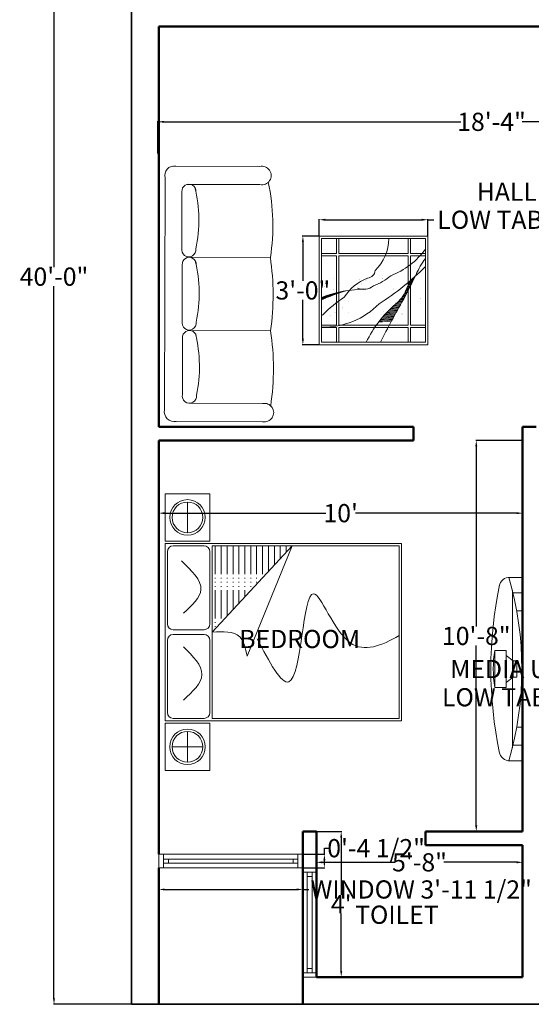
# Model space of a CAD drawing. Units: inches. Extents: x 134 to 568, y 15 to 554.
# Tile 1 of 7: x 134 to 303, y 45 to 369. Entities that reach past the tile are written whole.
import ezdxf

# ---------------------------------------------------------------- set-up
doc = ezdxf.new("R2010")
doc.units = ezdxf.units.IN
doc.header["$MEASUREMENT"] = 0
for name, color, linetype, lineweight in [('A-ANNO-DIMS', 2, 'Continuous', 18), ('A-AREA-IDEN', 7, 'Continuous', 25), ('A-EQPM', 8, 'Continuous', 18), ('A-FURN', 9, 'Continuous', 18), ('A-GLAZ', 4, 'Continuous', 18), ('A-WALL', 7, 'Continuous', 50), ('C-PROP', 7, 'Continuous', 35)]:
    doc.layers.add(name, color=color, linetype=linetype, lineweight=lineweight)
doc.styles.get("Standard").update_dxf_attribs({"font": 'arial.ttf'})
doc.dimstyles.get("Standard").update_dxf_attribs({"dimtxt": 6, "dimasz": 2, "dimexe": 0.18, "dimexo": 0.0625, "dimgap": 0.09, "dimtad": 0, "dimtih": 1, "dimtoh": 1, "dimdec": 0, "dimzin": 0, "dimdsep": 46, "dimlunit": 4, "dimtxsty": 'Standard', "dimcen": 0.09, "dimadec": 0, "dimazin": 0, "dimtfac": 1, "dimtdec": 0, "dimtofl": 0, "dimtmove": 0, "dimatfit": 3, "dimfxl": 1, "dimtolj": 1, "dimtzin": 0, "dimarcsym": 0})

# ---------------------------------------------------------------- blocks, each defined once
blk = doc.blocks.new('fdgchj')
for p, q in [((180.0833573093669, -8.682097346214732), (180.0833573093669, -13.18209734621473)), ((180.0833573093669, -8.682097346214732), (227.5833573093669, -8.682097346214716)), ((181.6833573093668, -8.682097346214732), (181.6833573093668, -13.18209734621473)), ((225.9833573093669, -8.682097346214716), (225.9833573093669, -13.18209734621463)), ((227.5833573093669, -8.682097346214716), (227.5833573093669, -13.18209734621463)), ((181.6833573093668, -10.28209734621472), (225.9833573093669, -10.28209734621471)), ((181.6833573093668, -11.58209734621473), (225.9833573093669, -11.58209734621464)), ((183.2833573093669, -10.28209734621472), (183.2833573093669, -11.58209734621473)), ((224.3833573093669, -10.28209734621471), (224.3833573093669, -11.58209734621464)), ((180.0833573093669, -13.18209734621473), (227.5833573093669, -13.18209734621463))]:
    blk.add_line(p, q)
blk = doc.blocks.new('*D9')
at = {"layer": 'A-ANNO-DIMS', "color": 0, "lineweight": -2, "transparency": 16777216}
for p, q in [((232.145857309367, 101.5821619144604), (240.4398249294156, 101.5821619144604)), ((240.2598249294155, 99.58216191446044), (240.2598249294155, 80.67216191446046)), ((240.2598249294156, 55.58216191446049), (240.2598249294155, 74.49216191446045)), ((232.1458573093669, 53.58216191446047), (240.4398249294156, 53.58216191446048))]:
    blk.add_line(p, q, dxfattribs=at)
at = {"layer": 'A-ANNO-DIMS', "color": 0, "transparency": 16777216}
for points in [[(239.9264915960822, 99.58216191446044), (240.5931582627489, 99.58216191446044), (240.2598249294155, 101.5821619144604)], [(239.9264915960822, 55.58216191446048), (240.5931582627489, 55.58216191446049), (240.2598249294156, 53.58216191446048)]]:
    blk.add_solid(points, dxfattribs=at)
at = {"layer": 'Defpoints', "color": 0, "transparency": 16777216}
for p in [(232.083357309367, 101.5821619144604), (232.0833573093669, 53.58216191446047), (240.2598249294156, 53.58216191446048)]:
    blk.add_point(p, dxfattribs=at)
at = {"layer": 'A-ANNO-DIMS', "color": 0, "transparency": 16777216, "insert": (240.2598249294155, 77.58216191446037), "char_height": 6, "attachment_point": 5}
blk.add_mtext("\\A1;4'", dxfattribs=at)
blk = doc.blocks.new('*D14')
at = {"layer": 'A-ANNO-DIMS', "color": 0, "lineweight": -2, "transparency": 16777216}
for p, q in [((300.0208573093672, 230.5821619144605), (284.6214758231763, 230.5821619144605)), ((284.8014758231764, 228.5821619144605), (284.8014758231764, 169.2355998407906)), ((284.8014758231764, 103.5821619144604), (284.8014758231764, 162.9287239881303)), ((300.020857309367, 101.5821619144604), (284.6214758231764, 101.5821619144604))]:
    blk.add_line(p, q, dxfattribs=at)
at = {"layer": 'A-ANNO-DIMS', "color": 0, "transparency": 16777216}
for points in [[(284.4681424898431, 228.5821619144605), (285.1348091565096, 228.5821619144605), (284.8014758231764, 230.5821619144605)], [(284.4681424898431, 103.5821619144604), (285.1348091565098, 103.5821619144604), (284.8014758231764, 101.5821619144604)]]:
    blk.add_solid(points, dxfattribs=at)
at = {"layer": 'Defpoints', "color": 0, "transparency": 16777216}
for p in [(300.0833573093672, 230.5821619144605), (284.8014758231764, 101.5821619144604), (300.083357309367, 101.5821619144604)]:
    blk.add_point(p, dxfattribs=at)
at = {"layer": 'A-ANNO-DIMS', "color": 0, "transparency": 16777216, "insert": (284.8014758231764, 166.0821619144603), "char_height": 6, "attachment_point": 5}
blk.add_mtext('\\A1;10\'-8"', dxfattribs=at)
blk = doc.blocks.new('*D15')
at = {"layer": 'A-ANNO-DIMS', "color": 0, "lineweight": -2, "transparency": 16777216}
for p, q in [((180.0833573093669, 230.5196619144604), (180.0833573093669, 206.3961685645716)), ((300.0833573093669, 230.5196619144604), (300.0833573093669, 206.3961685645716)), ((182.0833573093669, 206.5761685645716), (235.1843532165974, 206.5761685645716)), ((298.0833573093669, 206.5761685645716), (244.9823614021363, 206.5761685645716))]:
    blk.add_line(p, q, dxfattribs=at)
at = {"layer": 'A-ANNO-DIMS', "color": 0, "transparency": 16777216}
for points in [[(182.0833573093669, 206.909501897905), (182.0833573093669, 206.2428352312383), (180.0833573093669, 206.5761685645716)], [(298.0833573093669, 206.909501897905), (298.0833573093669, 206.2428352312383), (300.0833573093669, 206.5761685645716)]]:
    blk.add_solid(points, dxfattribs=at)
at = {"layer": 'Defpoints', "color": 0, "transparency": 16777216}
for p in [(180.0833573093669, 230.5821619144603), (300.0833573093669, 230.5821619144603), (300.0833573093669, 206.5761685645716)]:
    blk.add_point(p, dxfattribs=at)
at = {"layer": 'A-ANNO-DIMS', "color": 0, "transparency": 16777216, "insert": (240.0833573093669, 206.5761685645716), "char_height": 6, "attachment_point": 5}
blk.add_mtext("\\A1;10'", dxfattribs=at)
blk = doc.blocks.new('*D22')
at = {"layer": 'A-ANNO-DIMS', "color": 0, "lineweight": -2, "transparency": 16777216}
for p, q in [((179.8333573093669, 325.1446619144604), (179.8333573093669, 335.8252549678748)), ((181.8333573093669, 335.6452549678747), (279.7201649492031, 335.6452549678747)), ((397.8333573093669, 335.6452549678747), (299.9465496695306, 335.6452549678747)), ((399.8333573093669, 325.1446619144604), (399.8333573093669, 335.8252549678748))]:
    blk.add_line(p, q, dxfattribs=at)
at = {"layer": 'A-ANNO-DIMS', "color": 0, "transparency": 16777216}
for points in [[(181.8333573093669, 335.978588301208), (181.8333573093669, 335.3119216345414), (179.8333573093669, 335.6452549678747)], [(397.8333573093669, 335.978588301208), (397.8333573093669, 335.3119216345414), (399.8333573093669, 335.6452549678747)]]:
    blk.add_solid(points, dxfattribs=at)
at = {"layer": 'Defpoints', "color": 0, "transparency": 16777216}
for p in [(179.8333573093669, 335.6452549678747), (179.8333573093669, 325.0821619144604), (399.8333573093669, 325.0821619144604)]:
    blk.add_point(p, dxfattribs=at)
at = {"layer": 'A-ANNO-DIMS', "color": 0, "transparency": 16777216, "insert": (289.8333573093669, 335.6452549678747), "char_height": 6, "attachment_point": 5}
blk.add_mtext('\\A1;18\'-4"', dxfattribs=at)
blk = doc.blocks.new('dfghj')
h = blk.add_hatch()
h.set_pattern_fill('ACAD_ISO06W100', color=256, scale=0.5400000000000001, style=0)
h.set_pattern_definition([(0, (-45.65929459918516, 81.2680393364767), (0, 2.7), [12.96, -1.62, 0.27, -1.62, 0.27, -3.51]), (0, (-45.65929459918516, 81.2680393364767), (0, 2.7), [-18.36, 0.27, -1.62])])
h.paths.add_polyline_path([(495.420705400802, 683.3680393364771), (534.8407054008148, 646.8981935885663), (534.8407054008148, 683.3680393364771)])
for p, q in [((432.2407054008163, 704.9680393364765), (453.8407054008148, 704.9680393364765)), ((432.2407054008163, 704.9680393364765), (432.2407054008163, 684.4480393364788)), ((443.0407054008119, 701.7280393364721), (443.0407054008119, 687.6880393364768)), ((453.8407054008148, 704.9680393364765), (453.8407054008148, 684.4480393364788)), ((454.920705400802, 704.9680393364765), (454.920705400802, 596.9680393364765)), ((454.920705400802, 704.9680393364765), (535.920705400802, 704.9680393364765)), ((458.7007054008154, 703.8880393364766), (491.6407054008105, 703.8880393364766)), ((499.2007054008154, 703.8880393364766), (532.1407054008104, 703.8880393364766)), ((535.920705400802, 704.9680393364765), (535.920705400802, 596.9680393364765)), ((537.0007054008183, 704.9680393364765), (558.6007054008168, 704.9680393364765)), ((537.0007054008183, 704.9680393364765), (537.0007054008183, 684.4480393364788)), ((558.6007054008168, 704.9680393364765), (558.6007054008168, 684.4480393364788)), ((456.0007054008183, 701.1880393364767), (456.0007054008183, 687.1480393364795)), ((494.3407054008148, 701.1880393364767), (494.3407054008148, 687.1480393364795)), ((496.5007054008183, 701.1880393364767), (496.5007054008183, 687.1480393364795)), ((534.8407054008148, 701.1880393364767), (534.8407054008148, 687.1480393364795)), ((436.0207054008006, 694.7080393364744), (450.060705400816, 694.7080393364744)), ((540.7807054008099, 694.7080393364744), (554.8207054008035, 694.7080393364744)), ((432.2407054008163, 684.4480393364788), (453.8407054008148, 684.4480393364788)), ((458.7007054008154, 684.4480393364788), (491.6407054008105, 684.4480393364788)), ((499.2007054008154, 684.4480393364788), (532.1407054008104, 684.4480393364788)), ((537.0007054008183, 684.4480393364788), (558.6007054008168, 684.4480393364788)), ((456.0007054008183, 683.3680393364771), (456.0007054008183, 598.0480393364792)), ((456.0007054008183, 683.3680393364771), (534.8407054008148, 683.3680393364771)), ((495.420705400802, 683.3680393364771), (534.8407054008148, 646.8981935885663)), ((534.8407054008148, 683.3680393364771), (534.8407054008148, 598.0480393364792)), ((484.408206427508, 667.4334197787679), (534.8407054008148, 646.8981935885663)), ((456.0007054008183, 598.0480393364792), (534.8407054008148, 598.0480393364792)), ((454.920705400802, 596.9680393364765), (535.920705400802, 596.9680393364765))]:
    blk.add_line(p, q)
for centre, radius in [((443.0407054008119, 694.7080393364744), 8.1), ((443.0407054008119, 694.7080393364744), 7.020000000000001), ((547.800705400814, 694.7080393364744), 8.1), ((547.800705400814, 694.7080393364744), 7.020000000000001)]:
    blk.add_circle(centre, radius)
for centre, start, end in [((458.7007054008154, 701.1880393364767), 90, 180), ((491.6407054008105, 701.1880393364767), 0, 90), ((499.2007054008154, 701.1880393364767), 90, 180), ((532.1407054008104, 701.1880393364767), 0, 90), ((458.7007054008154, 687.1480393364795), 180, 270), ((491.6407054008105, 687.1480393364795), 270, 0), ((499.2007054008154, 687.1480393364795), 180, 270), ((532.1407054008104, 687.1480393364795), 270, 0)]:
    blk.add_arc(centre, 2.7, start, end)
for points, knots in [([(504.0873642108144, 696.4980886587387), (507.6478568661273, 692.6728528270118), (515.4209753861596, 684.3217580865917), (523.5337025619604, 692.8242520545471), (527.9303786509863, 697.4321614684745)], [0, 0, 0, 0, 13.36633595571319, 29.18082513308789, 29.18082513308789, 29.18082513308789, 29.18082513308789]), ([(464.3490068105038, 696.4980886587387), (468.2209746909002, 692.3657909551906), (476.1716983091387, 683.8805044125166), (484.4253643000896, 692.2199280984504), (488.6595307904953, 696.4980886587387)], [0, 0, 0, 0, 14.39706672085805, 29.56302891623292, 29.56302891623292, 29.56302891623292, 29.56302891623292]), ([(484.408206427508, 667.4334197787679), (487.9117447952648, 668.1466020798161), (496.0584065288031, 669.8049412646973), (495.6522124186928, 678.4441772793408), (495.420705400802, 683.3680393364771)], [0, 0, 0, 0, 9.565159985887036, 22.24154972850861, 22.24154972850861, 22.24154972850861, 22.24154972850861]), ([(492.399610210059, 662.8714304071177), (481.8503788042744, 657.380170521003), (453.252508497726, 642.4939354956872), (538.2357400049532, 642.1800857884786), (482.0018716074937, 623.4329456516238), (489.252723434607, 606.1225063401602), (493.8220791548028, 598.0480393364792)], [0, 0, 0, 0, 451.7784176077852, 1224.72435166985, 1743.990776893513, 2173.853229184429, 2173.853229184429, 2173.853229184429, 2173.853229184429])]:
    blk.add_open_spline(points, degree=3, knots=knots)
blk = doc.blocks.new('A$C78AE5658')
for p, q in [((1514.710072450669, 306.1060037219359), (1514.710072450669, 524.1059474034627)), ((1514.710072450669, 524.1059474034627), (2235.5102586675, 524.1059474034627)), ((2235.5102586675, 306.1060037219359), (2235.5102586675, 524.1059474034627)), ((98.35715676363363, 250.0000009555879), (98.35715676363363, 251.6199660723724)), ((98.35715676367727, 250.0000009555733), (98.35715676361907, 9.555878933e-07)), ((1514.710072450669, 306.1060037219359), (2235.5102586675, 306.1060037219359)), ((1613.280102290542, 306.1060037219359), (1715.729798347087, 167.9763742110153)), ((2136.940228827627, 306.1060037219359), (2034.490532771082, 167.9763742110153)), ((3648.35715676359, 250.0000009555733), (3648.35715676359, 251.6199660720231)), ((3648.35715676359, 9.555733413e-07), (3648.35715676359, 250.0000009555733)), ((3648.357156763605, 9.555733413e-07), (98.35715676363363, 9.555878933e-07)), ((348.3571567636482, 183.569161564541), (3398.357156763547, 183.5691615645264)), ((398.3571567636482, 9.555733413e-07), (398.3571567636482, 171.5666306721468)), ((748.357156763648, 9.555733413e-07), (748.357156763648, 99.2393274621354)), ((2034.490532771082, 167.9763742110153), (1715.729425914915, 167.9763742110153)), ((1715.729425914915, 167.9763742110153), (1715.729425914915, 97.54311758768019)), ((2034.490532771082, 97.54311758768019), (1715.729425914915, 97.54311758768019)), ((2034.490532771082, 167.9763742110153), (2034.490532771082, 97.54311758768019)), ((2998.35715676359, 9.555733413e-07), (2998.35715676359, 99.2393274621354)), ((3348.35715676359, 9.555733413e-07), (3348.35715676359, 171.5666306721468))]:
    blk.add_line(p, q)
blk.add_lwpolyline([(246.4015375078543, 431.9827464358895, -0.103184122095167), (3500.312775983877, 431.9827464432965, -0.103184122095167)], format="xyb")
for centre, radius, start, end in [((297.9418522906435, 238.7378345952966), 200, 98.46874505780073, 183.6930153877844), ((1875.110165559085, -1674.917347937364), 2228.360760865037, 80.69248372113285, 99.30751627886714), ((3448.772461236565, 238.7378345952966), 200, 356.3069846122155, 81.53125494219925), ((1873.357156763633, 6426.250000955618), 6426.25000000003, 253.9658138527447, 286.0341861472553)]:
    blk.add_arc(centre, radius, start, end)
blk = doc.blocks.new('A$C25EC1EFB')
h = blk.add_hatch()
h.set_pattern_fill('ANSI31', color=256, scale=2.508, angle=580, style=0)
h.set_pattern_definition([(94.99999999999984, (2801.512250582819, 4289.79602251789), (7.93259876143476, 0.6940124639253284), [])])
edge = h.paths.add_edge_path()
edge.add_ellipse((4084.490467177063, -2815.580363917667), major_axis=(-3872.16408689083, 3872.16408689083), ratio=0.9999999999995552, start_angle=340.89961915580596, end_angle=343.15488567038426, ccw=False)
edge.add_ellipse((1486.624568246823, 2293.159848771007), major_axis=(-194.6618757392838, 194.6618757392838), ratio=0.9999999999999246, start_angle=154.9056197196584, end_angle=183.4247301497222, ccw=False)
edge.add_ellipse((1687.117678346121, 1762.501521206774), major_axis=(-206.4950185728816, 206.4950185728816), ratio=0.999999999999898, start_angle=-23.5559095241906, end_angle=5.886608761987814)
edge.add_ellipse((823.8605303866296, 2467.162105106873), major_axis=(-581.4647167234576, 581.4647167234575), ratio=0.9999999999998493, start_angle=171.3363574034995, end_angle=185.7365630084011, ccw=False)
edge.add_line((1311.102457978037, 1804.744006331188), (1311.102457978037, 1908.515397835807))
edge.add_ellipse((-1407.416444189095, 7084.924681207201), major_axis=(4134.341428234145, 4134.341428234145), ratio=0.9999999999998351, start_angle=252.7073165240117, end_angle=254.8255249662156)
for p, q in [((1118.231915589249, 2219.932055225661), (1118.231915589242, 1300.332055225655)), ((2037.831915589246, 2219.932055225647), (1118.231915589249, 2219.932055225661)), ((2016.931915589244, 2199.032055225638), (1139.131915589243, 2199.032055225638)), ((1139.131915589243, 2199.032055225638), (1139.131915589243, 1321.232055225664)), ((1264.531915589245, 2199.032055225638), (1264.531915589245, 2073.63205522563)), ((1285.431915589246, 2199.032055225638), (1285.431915589246, 2073.63205522563)), ((1870.631915589243, 2199.032055225638), (1870.631915589243, 2073.632055225644)), ((1891.531915589245, 2199.032055225638), (1891.531915589245, 2073.632055225644)), ((2016.931915589244, 2199.032055225638), (2016.931915589244, 1321.23205522565)), ((2037.831915589246, 2219.932055225647), (2037.831915589246, 1300.332055225655)), ((1264.531915589245, 2073.63205522563), (1139.131915589243, 2073.632055225644)), ((1264.531915589245, 2052.732055225635), (1139.131915589243, 2052.732055225664)), ((1264.531915589245, 2052.732055225635), (1264.531915589245, 1467.532055225652)), ((1870.631915589243, 2073.632055225644), (1285.431915589246, 2073.63205522563)), ((1870.631915589243, 2052.73205522565), (1285.431915589246, 2052.732055225635)), ((1285.431915589246, 2052.732055225635), (1285.431915589246, 1467.532055225652)), ((1870.631915589243, 2052.73205522565), (1870.631915589243, 1467.532055225652)), ((2016.931915589244, 2073.632055225658), (1891.531915589245, 2073.632055225644)), ((1891.531915589245, 2052.73205522565), (1891.531915589245, 1467.532055225652)), ((2016.931915589244, 2052.73205522565), (1891.531915589245, 2052.73205522565)), ((1569.58961247749, 1498.845113355761), (1568.886649074042, 1506.88002182413)), ((1573.215999468995, 1518.30467450877), (1573.064505181503, 1520.03626213839)), ((1264.531915589245, 1467.532055225667), (1139.131915589243, 1467.532055225667)), ((1264.531915589245, 1446.632055225658), (1139.131915589243, 1446.632055225658)), ((1264.531915589245, 1446.632055225658), (1264.531915589245, 1321.23205522565)), ((1870.631915589243, 1467.532055225652), (1285.431915589246, 1467.532055225667)), ((1870.631915589243, 1446.632055225658), (1285.431915589246, 1446.632055225658)), ((1285.431915589246, 1446.632055225658), (1285.431915589246, 1321.23205522565)), ((1541.818491434993, 1389.905000426101), (1539.119938526573, 1420.749601311116)), ((1545.9666700701, 1403.400455801595), (1543.422872825396, 1432.476191356145)), ((1550.066663663807, 1417.446668720506), (1547.710096352946, 1444.382356338588)), ((1554.112776362645, 1432.108743085911), (1551.980974986758, 1456.475344311409)), ((1558.098049746682, 1447.466214001491), (1556.234828786708, 1468.762927025651)), ((1562.013830635669, 1463.617987770158), (1560.470927201475, 1481.253454721161)), ((1565.849127400865, 1480.689699283357), (1564.688483608976, 1493.955918529544)), ((1870.631915589243, 1446.632055225658), (1870.631915589243, 1321.23205522565)), ((2016.931915589244, 1467.532055225652), (1891.531915589245, 1467.532055225652)), ((1891.531915589245, 1446.632055225658), (1891.531915589245, 1321.23205522565)), ((2016.931915589244, 1446.632055225658), (1891.531915589245, 1446.632055225658)), ((1510.524449703889, 1321.232055225664), (1508.604887871583, 1343.172747367374)), ((1515.85332769347, 1321.232055225664), (1513.003113907138, 1353.810147877557)), ((1520.497301609701, 1329.060544606509), (1517.389086063931, 1364.587610862924)), ((1524.828260129872, 1340.466816335822), (1521.762395858635, 1375.50980530923)), ((1529.128590691436, 1352.223167233933), (1526.122610320157, 1386.58168009873)), ((1533.395763262031, 1364.358515703112), (1530.469269874078, 1397.808488191054)), ((1537.626860969483, 1376.906201744794), (1534.801885985626, 1409.195813564198)), ((2037.831915589246, 1300.332055225655), (1118.231915589242, 1300.332055225655)), ((2016.931915589244, 1321.23205522565), (1139.131915589243, 1321.232055225664)), ((1499.866693724727, 1321.232055225664), (1499.773196894175, 1322.300728889044)), ((1505.195571714308, 1321.23205522565), (1504.194793856486, 1332.670998484005))]:
    blk.add_line(p, q)
at = {"const_width": 2.09}
for points in [[(1511.151005801041, 2155.427417849518, -1), (1511.151005801041, 2153.337417849522, -1)], [(1749.963977974703, 2129.419879811459, -1), (1749.963977974703, 2127.329879811463, -1)], [(1378.464403896922, 2001.982938292022, -1), (1378.464403896922, 1999.892938292025, -1)], [(1378.464403896922, 2000.937938292024, -1), (1378.464403896922, 1998.847938292026, -1)], [(1472.141222166467, 1950.101574691951, -1), (1472.141222166467, 1948.011574691955, -1)], [(1589.664228032883, 1926.272639169089, -1), (1589.664228032883, 1924.182639169077, -1)], [(1396.649697045645, 1848.538458734525, -1), (1396.649697045645, 1846.448458734528, -1)], [(1498.485842016862, 1893.112440112549, -1), (1498.485842016862, 1891.022440112552, -1)], [(1677.799055322533, 1835.246250902906, -1), (1677.799055322533, 1833.15625090291, -1)], [(1661.635412078192, 1692.493220240234, -1), (1661.635412078192, 1690.403220240223, -1)], [(1682.418605074026, 1710.698501999875, -1), (1682.418605074026, 1708.608501999864, -1)], [(1632.519993189891, 1660.01154033171, -1), (1632.519993189891, 1657.921540331714, -1)], [(1672.027005685611, 1645.679651771737, -1), (1672.027005685611, 1643.589651771741, -1)], [(1390.689109610934, 1549.797216376151, -1), (1390.689109610934, 1547.707216376155, -1)], [(1484.978268723158, 1546.850996961155, -1), (1484.978268723158, 1544.760996961158, -1)], [(1519.878047569999, 1513.762184183615, -1), (1519.878047569999, 1511.672184183619, -1)], [(1394.744337709578, 1434.839303017281, -1), (1394.744337709578, 1432.74930301727, -1)], [(1435.398901256181, 1495.038386561347, -1), (1435.398901256181, 1492.948386561351, -1)], [(1587.165183262217, 1425.04444594484, -1), (1587.165183262217, 1422.954445944844, -1)], [(1638.254319235255, 1463.626875239402, -1), (1638.254319235255, 1461.536875239391, -1)], [(1675.222175186443, 1421.779486743347, -1), (1675.222175186443, 1419.689486743351, -1)], [(1675.788258493603, 1422.657879986356, -1), (1675.788258493603, 1420.567879986345, -1)], [(1365.392005141164, 1392.394905260015, -1), (1365.392005141164, 1390.304905260018, -1)], [(1370.896625781812, 1333.067117625229, -1), (1370.896625781812, 1330.977117625232, -1)], [(1613.584636758898, 1347.361959619193, -1), (1613.584636758898, 1345.271959619196, -1)], [(1639.675595830262, 1353.891867756152, -1), (1639.675595830262, 1351.801867756156, -1)]]:
    blk.add_lwpolyline(points, format="xyb", close=True, dxfattribs=at)
for centre, radius, start, end in [((3333.68451552435, 627.3607967675852), 2209.54164879086, 134.6725360764692, 147.7436105193565), ((2287.848786312694, 1688.392912899486), 624.2670274309789, 125.1781643370384, 159.5766212149076), ((1462.653166443046, 2709.567626046374), 640.2705249755662, 292.8904712152515, 307.0626715443762), ((4084.490467176721, -2815.580363917798), 5476.066967415318, 115.6772969660199, 118.1548856704495), ((1486.624568246801, 2293.159848771022), 275.2934647474958, 289.9056197197872, 318.4247301496573), ((-2476.242387987366, 8989.86383017015), 8031.077363206627, 296.7547849003873, 299.6814985470403), ((1687.117678346143, 1762.501521206774), 292.0280558282651, 111.4440904757719, 140.8866087620124), ((751.7750952702208, 2534.062472635524), 920.4881034674244, 294.8861636343854, 320.3521788954757), ((2051.740526511305, 1602.642054351665), 462.5051862275705, 138.9735804164881, 160.2295429731453), ((2014.166362558564, 1518.116840648719), 370.3125627779616, 89.60713639418466, 136.3509345096815), ((1916.655318256047, 1341.313739382756), 648.3552410927683, 134.1383379809644, 181.6847040310653), ((1726.67177394053, 1673.301525916809), 139.6326613666137, 142.0948538523169, 200.8895128689712), ((1752.222980010354, 1704.369846744921), 69.61106324809847, 94.95105755802923, 174.8766543317414), ((576.7142338831854, 1693.940106953196), 1011.861440092256, 338.386783207812, 0.0010917430398909), ((1322.831429736014, 1838.987718223034), 381.1559142689087, 301.1293017828129, 340.1644872338225), ((792.9020607460498, 1960.337764563381), 853.7319657820956, 312.6112985239825, 328.3781661717325), ((-408.4163850434979, 2142.027900565321), 2076.810081976653, 336.7203354898851, 342.6666348099279), ((1307.752931048004, 1350.181809599417), 65.70312471435534, 333.8568999860387, 343.9551289370007)]:
    blk.add_arc(centre, radius, start, end)
blk = doc.blocks.new('*D33')
at = {"layer": 'A-ANNO-DIMS', "color": 0, "lineweight": -2, "transparency": 16777216}
for p, q in [((232.0833573093669, 101.5196619144604), (232.0833573093669, 91.22939516274556)), ((300.0833573093669, 97.01966191446039), (300.0833573093669, 91.22939516274556)), ((234.0833573093669, 91.40939516274555), (258.0185960542509, 91.40939516274555)), ((298.0833573093669, 91.40939516274555), (274.1481185644829, 91.40939516274555))]:
    blk.add_line(p, q, dxfattribs=at)
at = {"layer": 'A-ANNO-DIMS', "color": 0, "transparency": 16777216}
for points in [[(234.0833573093669, 91.7427284960789), (234.0833573093669, 91.07606182941223), (232.0833573093669, 91.40939516274555)], [(298.0833573093669, 91.7427284960789), (298.0833573093669, 91.07606182941223), (300.0833573093669, 91.40939516274555)]]:
    blk.add_solid(points, dxfattribs=at)
at = {"layer": 'Defpoints', "color": 0, "transparency": 16777216}
for p in [(232.0833573093669, 101.5821619144604), (300.0833573093669, 97.08216191446037), (300.0833573093669, 91.40939516274555)]:
    blk.add_point(p, dxfattribs=at)
at = {"layer": 'A-ANNO-DIMS', "color": 0, "transparency": 16777216, "insert": (266.0833573093669, 91.40939516274555), "char_height": 6, "attachment_point": 5}
blk.add_mtext('\\A1;5\'-8"', dxfattribs=at)
blk = doc.blocks.new('SOFA-3-SEAT')
for p, q in [((2.639539900301173, 84.33324550660927, -275.7706107739931), (31.48293072343935, 84.25018466807978, -275.7706107739931)), ((0.0383790449484991, 3.974159020291153, -275.7706107739931), (0.3339295813419483, 80.44811578913232, -275.7706107739931)), ((7.498200915528144, 78.33324550660927, -275.7706107739931), (31.56791808250259, 78.25018466807978, -275.7706107739931)), ((5.843710623688679, 57.34215320189196, -275.7706107739931), (5.843710623688679, 75.93023828611786, -275.7706107739931)), ((5.843710623688679, 57.34215320189196, -275.7706107739931), (5.843710623688679, 75.93023828611786, -275.7706107739931)), ((34.99945515191198, 54.21758312230394, -275.7706107739931), (8.231751979335826, 54.28260851868344, -275.7706107739931)), ((5.943773992104809, 33.20240762962658, -275.7706107739931), (5.943773992104837, 51.79049271384883, -275.7706107739931)), ((5.943773992104809, 33.20240762962658, -275.7706107739931), (5.943773992104837, 51.79049271385611, -275.7706107739931)), ((35.09951852032811, 30.07783755003129, -275.7706107739931), (8.331815347751956, 30.14286294641079, -275.7706107739931)), ((6.043837360520967, 9.062662057353918, -275.7706107739931), (6.043837360520967, 27.65074714157618, -275.7706107739931)), ((6.043837360520967, 9.062662057353918, -275.7706107739931), (6.043837360520967, 27.65074714157618, -275.7706107739931)), ((8.302397746832696, 6.142582730023605, -275.7706107739931), (32.4491326919013, 6.059521891490476, -275.7706107739931)), ((3.975506222290107, 0.1425827300236051, -275.7706107739931), (32.4491326919013, 0.0595218914904763, -275.7706107739931))]:
    blk.add_line(p, q)
for centre, radius, start, end in [((3.220976162505252, 81.35906493094171, -275.7706107739931), 3.02735301884233, 78.91083061777086, 197.5120367194869), ((32.20255676183283, 81.25977594989763, -275.7706107739931), 3.075777289872148, 258.0923749518217, 103.5306555133332), ((8.131688610919667, 76.12601528668618, -275.7706107739931), 2.296338804262066, 355.1092454701771, 184.8907545298229), ((-31.3836276940348, 64.73871829630025, -275.7706107739931), 67.21166545684105, 350.9940323093792, 12.25610082943838), ((-33.55016406365772, 66.49239086433681, -275.7706107739931), 44.97131277140765, 347.8856334289421, 13.9133261029634), ((8.103939744214443, 56.75685568044809, -275.7706107739931), 2.334782402231908, 165.4818835729592, 7.325225020201399), ((8.231751979335826, 51.98626971442445, -275.7706107739931), 2.296338804262066, 355.1092454701771, 184.8907545298229), ((-33.45010069524156, 42.35264529206415, -275.7706107739931), 44.97131277140765, 347.8856334289421, 13.9133261029634), ((-49.15139397142789, 41.79868330390036, -275.7706107739931), 85.06229764636532, 352.0799408120631, 8.39505804799601), ((8.204003112630573, 32.61711010817544, -275.7706107739931), 2.334782402231908, 165.4818835729592, 7.325225020201399), ((8.331815347751956, 27.84652414215179, -275.7706107739931), 2.296338804262066, 355.1092454701771, 184.8907545298229), ((-49.05133060301174, 17.65893773163134, -275.7706107739931), 85.06229764636532, 351.661265989887, 8.39505804799601), ((-33.3500373268254, 18.21289971979877, -275.7706107739931), 44.97131277140765, 347.8856334289421, 13.9133261029634), ((8.304066481017628, 8.477364535906418, -275.7706107739931), 2.334782402231908, 165.4818835729592, 7.325225020201399), ((3.371955953108965, 3.460987091163588, -275.7706107739931), 3.37284456082161, 171.2485666807343, 280.3082563582749), ((33.05221387278999, 3.059521891490476, -275.7706107739931), 3.060017469021007, 258.6334958280249, 101.366504171975)]:
    blk.add_arc(centre, radius, start, end)
blk = doc.blocks.new('*D38')
at = {"layer": 'A-ANNO-DIMS', "color": 0, "lineweight": -2, "transparency": 16777216}
for p, q in [((316.172408782906, 185.5132349532936), (325.3973721430653, 185.5132349532937)), ((325.2173721430653, 183.5132349532937), (325.2173721430653, 158.3473429887794)), ((325.2173721430653, 126.7968125522324), (325.2173721430653, 151.9627045167466)), ((316.172408782906, 124.7968125522324), (325.3973721430654, 124.7968125522324))]:
    blk.add_line(p, q, dxfattribs=at)
at = {"layer": 'A-ANNO-DIMS', "color": 0, "transparency": 16777216}
for points in [[(324.884038809732, 183.5132349532937), (325.5507054763986, 183.5132349532937), (325.2173721430653, 185.5132349532937)], [(324.884038809732, 126.7968125522324), (325.5507054763987, 126.7968125522324), (325.2173721430653, 124.7968125522324)]]:
    blk.add_solid(points, dxfattribs=at)
at = {"layer": 'Defpoints', "color": 0, "transparency": 16777216}
for p in [(316.109908782906, 185.5132349532936), (325.2173721430653, 185.5132349532937), (316.109908782906, 124.7968125522324)]:
    blk.add_point(p, dxfattribs=at)
at = {"layer": 'A-ANNO-DIMS', "color": 0, "transparency": 16777216, "insert": (325.2173721430653, 155.1550237527629), "char_height": 6, "attachment_point": 5}
blk.add_mtext('\\A1;MEDIA UNIT 5\'-0 1/2" TYP.', dxfattribs=at)
blk = doc.blocks.new('*D46')
at = {"layer": 'A-ANNO-DIMS', "color": 0, "lineweight": -2, "transparency": 16777216}
for p, q in [((232.9940473437014, 298.0284180589613), (232.9940473437014, 303.5240191414689)), ((234.9940473437014, 303.3440191414689), (266.8480545604188, 303.3440191414689)), ((268.8480545604188, 298.0284180589613), (268.8480545604188, 303.5240191414689)), ((268.8480545604188, 303.3440191414689), (270.8480545604188, 303.3440191414689))]:
    blk.add_line(p, q, dxfattribs=at)
at = {"layer": 'A-ANNO-DIMS', "color": 0, "transparency": 16777216}
for points in [[(234.9940473437014, 303.6773524748022), (234.9940473437014, 303.0106858081356), (232.9940473437014, 303.3440191414689)], [(266.8480545604188, 303.6773524748022), (266.8480545604188, 303.0106858081356), (268.8480545604188, 303.3440191414689)]]:
    blk.add_solid(points, dxfattribs=at)
at = {"layer": 'Defpoints', "color": 0, "transparency": 16777216}
for p in [(268.8480545604188, 303.3440191414689), (232.9940473437014, 297.9659180589613), (268.8480545604188, 297.9659180589613)]:
    blk.add_point(p, dxfattribs=at)
at = {"layer": 'A-ANNO-DIMS', "color": 0, "transparency": 16777216, "insert": (303.9319154062578, 303.3440191414689), "char_height": 6, "attachment_point": 5}
blk.add_mtext('\\A1;LOW TABLE 3\'-0"', dxfattribs=at)
blk = doc.blocks.new('*D47')
at = {"layer": 'A-ANNO-DIMS', "color": 0, "lineweight": -2, "transparency": 16777216}
for p, q in [((232.9315473437015, 297.9659180589614), (227.4359462611939, 297.9659180589614)), ((227.615946261194, 295.9659180589614), (227.615946261194, 283.1943987616532)), ((227.615946261194, 264.111910842244), (227.615946261194, 276.8834301395522)), ((232.9315473437015, 262.111910842244), (227.4359462611939, 262.111910842244))]:
    blk.add_line(p, q, dxfattribs=at)
at = {"layer": 'A-ANNO-DIMS', "color": 0, "transparency": 16777216}
for points in [[(227.2826129278606, 295.9659180589614), (227.9492795945273, 295.9659180589614), (227.615946261194, 297.9659180589614)], [(227.2826129278606, 264.111910842244), (227.9492795945273, 264.111910842244), (227.615946261194, 262.111910842244)]]:
    blk.add_solid(points, dxfattribs=at)
at = {"layer": 'Defpoints', "color": 0, "transparency": 16777216}
for p in [(227.615946261194, 297.9659180589614), (232.9940473437015, 297.9659180589614), (232.9940473437015, 262.111910842244)]:
    blk.add_point(p, dxfattribs=at)
at = {"layer": 'A-ANNO-DIMS', "color": 0, "transparency": 16777216, "insert": (227.615946261194, 280.0389144506026), "char_height": 6, "attachment_point": 5}
blk.add_mtext('\\A1;3\'-0"', dxfattribs=at)
blk = doc.blocks.new('*D48')
at = {"layer": 'A-ANNO-DIMS', "color": 0, "lineweight": -2, "transparency": 16777216}
for p, q in [((340.5750090510671, 150.2827316451021), (340.5750090510671, 145.672982833064)), ((370.523334464654, 150.2827316451021), (370.523334464654, 145.672982833064)), ((340.5750090510671, 145.852982833064), (338.5750090510671, 145.852982833064)), ((368.523334464654, 145.852982833064), (342.5750090510671, 145.852982833064))]:
    blk.add_line(p, q, dxfattribs=at)
at = {"layer": 'A-ANNO-DIMS', "color": 0, "transparency": 16777216}
for points in [[(342.5750090510671, 146.1863161663974), (342.5750090510671, 145.5196494997307), (340.5750090510671, 145.852982833064)], [(368.523334464654, 146.1863161663974), (368.523334464654, 145.5196494997307), (370.523334464654, 145.852982833064)]]:
    blk.add_solid(points, dxfattribs=at)
at = {"layer": 'Defpoints', "color": 0, "transparency": 16777216}
for p in [(340.5750090510671, 150.3452316451021), (370.523334464654, 150.3452316451021), (340.5750090510671, 145.852982833064)]:
    blk.add_point(p, dxfattribs=at)
at = {"layer": 'A-ANNO-DIMS', "color": 0, "transparency": 16777216, "insert": (305.4911482052281, 145.852982833064), "char_height": 6, "attachment_point": 5}
blk.add_mtext('\\A1;LOW TABLE 2\'-6"', dxfattribs=at)
blk = doc.blocks.new('*D52')
at = {"layer": 'A-ANNO-DIMS', "color": 0, "lineweight": -2, "transparency": 16777216}
for p, q in [((180.0833573093669, 89.51966191446027), (180.0833573093669, 82.27716191446027)), ((227.5833573093669, 89.51966191446027), (227.5833573093669, 82.27716191446027)), ((182.0833573093669, 82.45716191446026), (225.5833573093669, 82.45716191446026)), ((227.5833573093669, 82.45716191446026), (229.5833573093669, 82.45716191446026))]:
    blk.add_line(p, q, dxfattribs=at)
at = {"layer": 'A-ANNO-DIMS', "color": 0, "transparency": 16777216}
for points in [[(182.0833573093669, 82.7904952477936), (182.0833573093669, 82.12382858112694), (180.0833573093669, 82.45716191446026)], [(225.5833573093669, 82.7904952477936), (225.5833573093669, 82.12382858112694), (227.5833573093669, 82.45716191446026)]]:
    blk.add_solid(points, dxfattribs=at)
at = {"layer": 'Defpoints', "color": 0, "transparency": 16777216}
for p in [(180.0833573093669, 89.58216191446027), (227.5833573093669, 89.58216191446027), (227.5833573093669, 82.45716191446026)]:
    blk.add_point(p, dxfattribs=at)
at = {"layer": 'A-ANNO-DIMS', "color": 0, "transparency": 16777216, "insert": (266.6453900515224, 82.45716191446026), "char_height": 6, "attachment_point": 5}
blk.add_mtext('\\A1;WINDOW 3\'-11 1/2"', dxfattribs=at)
blk = doc.blocks.new('*D53')
at = {"layer": 'A-ANNO-DIMS', "color": 0, "lineweight": -2, "transparency": 16777216}
for p, q in [((234.7083573093671, 94.08216191446031), (234.7083573093671, 96.08216191446031)), ((234.7083573093671, 96.08216191446031), (236.7083573093671, 96.08216191446031)), ((227.645857309367, 94.08216191446031), (234.8883573093671, 94.08216191446031)), ((234.7083573093671, 91.5821619144603), (234.7083573093671, 92.08216191446031)), ((227.645857309367, 89.5821619144603), (234.8883573093671, 89.5821619144603))]:
    blk.add_line(p, q, dxfattribs=at)
at = {"layer": 'A-ANNO-DIMS', "color": 0, "transparency": 16777216}
for points in [[(234.3750239760338, 92.08216191446031), (235.0416906427005, 92.08216191446031), (234.7083573093671, 94.08216191446031)], [(234.3750239760338, 91.5821619144603), (235.0416906427005, 91.5821619144603), (234.7083573093671, 89.5821619144603)]]:
    blk.add_solid(points, dxfattribs=at)
at = {"layer": 'Defpoints', "color": 0, "transparency": 16777216}
for p in [(227.583357309367, 94.08216191446031), (234.7083573093671, 94.08216191446031), (227.583357309367, 89.5821619144603)]:
    blk.add_point(p, dxfattribs=at)
at = {"layer": 'A-ANNO-DIMS', "color": 0, "transparency": 16777216, "insert": (251.7635687691215, 96.08216191446024), "char_height": 6, "attachment_point": 5}
blk.add_mtext('\\A1;0\'-4 1/2"', dxfattribs=at)
blk = doc.blocks.new('*D58')
at = {"layer": 'A-ANNO-DIMS', "color": 0, "lineweight": -2, "transparency": 16777216}
for p, q in [((171.020857, 524.5821620000002), (145.353357, 524.5821620000002)), ((145.533357, 522.5821620000003), (145.5333570000001, 287.7355999263303)), ((145.5333570000001, 46.582162), (145.5333570000001, 281.42872407367)), ((171.020857, 44.58216200000001), (145.3533570000001, 44.58216200000001))]:
    blk.add_line(p, q, dxfattribs=at)
at = {"layer": 'A-ANNO-DIMS', "color": 0, "transparency": 16777216}
for points in [[(145.2000236666667, 522.5821620000003), (145.8666903333334, 522.5821620000003), (145.533357, 524.5821620000002)], [(145.2000236666668, 46.582162), (145.8666903333335, 46.582162), (145.5333570000001, 44.58216200000001)]]:
    blk.add_solid(points, dxfattribs=at)
at = {"layer": 'Defpoints', "color": 0, "transparency": 16777216}
for p in [(145.533357, 524.5821620000002), (171.083357, 524.5821620000002), (171.083357, 44.58216200000001)]:
    blk.add_point(p, dxfattribs=at)
at = {"layer": 'A-ANNO-DIMS', "color": 0, "transparency": 16777216, "insert": (145.5333570000001, 284.582162), "char_height": 6, "attachment_point": 5}
blk.add_mtext('\\A1;40\'-0"', dxfattribs=at)

msp = doc.modelspace()

# ---------------------------------------------------------------- linework, layer by layer
at = {"layer": 'A-GLAZ'}
for p, q in [((227.5833573093669, 89.58216191446044), (232.0833573093668, 89.58216191446044)), ((227.5833573093668, 53.58216191446046), (227.5833573093669, 89.58216191446044)), ((227.5833573093669, 88.18216191446044), (232.0833573093668, 88.18216191446044)), ((228.9833573093668, 54.98216191446045), (228.9833573093669, 88.18216191446044)), ((230.6833573093669, 88.18216191446044), (230.6833573093668, 54.98216191446045)), ((232.0833573093669, 89.58216191446044), (232.0833573093668, 53.58216191446036)), ((228.9833573093669, 86.78216191446042), (230.6833573093669, 86.78216191446042)), ((230.6833573093668, 56.38216191446046), (228.9833573093668, 56.38216191446046)), ((232.0833573093668, 54.98216191446045), (227.5833573093668, 54.98216191446046)), ((232.0833573093668, 53.58216191446045), (227.5833573093668, 53.58216191446046))]:
    msp.add_line(p, q, dxfattribs=at)
at = {"layer": 'A-WALL'}
for p, q in [((180.0833573093669, 367.0821619144604), (180.0833573093669, 235.0821619144604)), ((180.0833573093669, 367.0821619144604), (316.5833573093669, 367.0821619144604)), ((180.0833573093669, 235.0821619144603), (264.0833573093671, 235.0821619144604)), ((264.0833573093671, 235.0821619144603), (264.0833573093671, 230.5821619144604)), ((300.0833573093671, 235.0821619144603), (300.0833573093669, 101.5821619144603)), ((300.0833573093671, 235.0821619144604), (304.5833573093669, 235.0821619144604)), ((180.0833573093669, 230.5821619144603), (264.0833573093672, 230.5821619144603)), ((180.0833573093669, 230.5821619144604), (180.0833573093668, 94.08216191446034)), ((227.5833573093669, 101.5821619144604), (227.5833573093668, 44.58216191446036)), ((227.5833573093669, 101.5821619144604), (232.0833573093669, 101.5821619144604)), ((268.0833573093669, 101.5821619144604), (300.0833573093669, 101.5821619144603)), ((268.0833573093669, 97.08216191446037), (300.0833573093669, 97.08216191446037)), ((300.0833573093669, 97.08216191446037), (300.0833573093668, 53.58216191446037)), ((180.0833573093668, 89.58216191446036), (180.0833573093669, 44.58216191446035)), ((232.0833573093668, 53.58216191446036), (300.0833573093668, 53.58216191446036))]:
    msp.add_line(p, q, dxfattribs=at)
for points in [[(232.0833573093669, 101.5821619144604), (232.0833573093668, 53.58216191446045)], [(268.0833573093669, 101.5821619144604), (268.0833573093669, 97.08216191446039)]]:
    msp.add_lwpolyline(points, dxfattribs=at)
at = {"layer": 'C-PROP'}
for p, q in [((171.0833573093669, 524.5821619144602), (171.0833573093669, 44.58216191446036)), ((171.0833573093669, 44.58216191446036), (531.0833573093669, 44.58216191446036))]:
    msp.add_line(p, q, dxfattribs=at)

# ---------------------------------------------------------------- block references
at = {"layer": 'A-EQPM', "xscale": 0.0170389131376971, "yscale": 0.0170389131376971, "zscale": 0.0170389131376971, "rotation": 90}
msp.add_blockref('A$C78AE5658', (299.8328734942244, 123.2350538827847), dxfattribs=at)
at = {"layer": 'A-FURN'}
msp.add_blockref('SOFA-3-SEAT', (181.887, 236.678), dxfattribs=at)
for name, p, xscale, yscale, zscale, rotation in [('A$C25EC1EFB', (182.2957927849917, 218.5135037396991), -0.0389886985827721, 0.0389886985827721, 0.0389886985827721, 270), ('dfghj', (691.3288752872245, -190.4894172478537), 0.7222806032890517, 0.7222806032890517, 0.7222806032890517, 90)]:
    msp.add_blockref(name, p, dxfattribs=dict(at, xscale=xscale, yscale=yscale, zscale=zscale, rotation=rotation))
at = {"layer": 'A-GLAZ'}
msp.add_blockref('fdgchj', (0, 102.764259260675), dxfattribs=at)

# ---------------------------------------------------------------- texts
at = {"layer": 'A-AREA-IDEN', "char_height": 6, "attachment_point": 1}
for s, width, insert in [('\\pxqc;HALL', 44.02085638939752, (272.8699323625169, 315.5900887416365)), ('BEDROOM', 59.5758364165049, (206.6359490243558, 168.0686458947493)), ('TOILET', 41.27017472680563, (244.836678575326, 77.12186031772944))]:
    msp.add_mtext_dynamic_manual_height_columns(s, width=width, gutter_width=30, heights=[0], dxfattribs=dict(at, insert=insert))

# ---------------------------------------------------------------- dimensions: what is measured, and where the dimension line sits
at = {"layer": 'A-ANNO-DIMS'}
for base, p1, p2, override, picture, middle in [((145.533357, 524.5821620000002), (171.083357, 44.58216199999999), (171.083357, 524.582162), {"dimdec": 1, "dimlfac": 1, "dimrnd": 0, "dimzin": 1, "dimdsep": 46, "dimlunit": 4, "dimfrac": 2}, '*D58', (145.5333570000001, 284.582162)), ((227.615946261194, 297.9659180589614), (232.9940473437014, 262.1119108422439), (232.9940473437014, 297.9659180589613), {"dimdec": 1, "dimlfac": 1, "dimrnd": 0, "dimzin": 1, "dimdsep": 46, "dimlunit": 4, "dimfrac": 2}, '*D47', (227.615946261194, 280.0389144506026)), ((234.7083573093671, 94.08216191446031), (227.5833573093669, 89.58216191446027), (227.5833573093669, 94.08216191446029), {"dimdec": 1, "dimlfac": 1, "dimrnd": 0, "dimzin": 1, "dimdsep": 46, "dimlunit": 4, "dimfrac": 2}, '*D53', (251.7635687691215, 96.08216191446024)), ((240.2598249294156, 53.58216191446048), (232.0833573093669, 101.5821619144604), (232.0833573093668, 53.58216191446045), {"dimclrd": 0, "dimclre": 0, "dimclrt": 0}, '*D9', (240.2598249294155, 77.58216191446037))]:
    dim = msp.add_linear_dim(base=base, p1=p1, p2=p2, angle=90, dimstyle='Standard', override=override, dxfattribs=at)
    dim.commit()
    dim.dimension.update_dxf_attribs({"geometry": picture, "text_midpoint": middle})
for base, p1, p2, picture, middle in [((179.8333573093669, 335.6452549678747), (399.8333573093669, 325.0821619144604), (179.8333573093669, 325.0821619144604), '*D22', (289.8333573093669, 335.6452549678747)), ((300.0833573093669, 206.5761685645716), (180.0833573093669, 230.5821619144603), (300.0833573093669, 230.5821619144603), '*D15', (240.0833573093669, 206.5761685645716)), ((300.0833573093669, 91.40939516274555), (232.0833573093669, 101.5821619144604), (300.0833573093669, 97.08216191446037), '*D33', (266.0833573093669, 91.40939516274555))]:
    dim = msp.add_linear_dim(base=base, p1=p1, p2=p2, dimstyle='Standard', override={"dimclrd": 0, "dimclre": 0, "dimclrt": 0}, dxfattribs=at)
    dim.commit()
    dim.dimension.update_dxf_attribs({"geometry": picture, "text_midpoint": middle})
for base, p1, p2, text, picture, middle in [((268.8480545604188, 303.3440191414689), (232.9940473437014, 297.9659180589613), (268.8480545604188, 297.9659180589613), 'LOW TABLE <>', '*D46', (303.9319154062578, 303.3440191414689)), ((227.5833573093669, 82.45716191446026), (180.0833573093669, 89.58216191446027), (227.5833573093669, 89.58216191446027), 'WINDOW <>', '*D52', (266.6453900515224, 82.45716191446026))]:
    dim = msp.add_linear_dim(base=base, p1=p1, p2=p2, text=text, dimstyle='Standard', override={"dimdec": 1, "dimlfac": 1, "dimrnd": 0, "dimzin": 1, "dimdsep": 46, "dimlunit": 4, "dimfrac": 2}, dxfattribs=at)
    dim.commit()
    dim.dimension.update_dxf_attribs({"geometry": picture, "text_midpoint": middle})
for base, p1, p2, angle, text, override, picture, middle in [((284.8014758231764, 101.5821619144604), (300.083357309367, 230.5821619144604), (300.0833573093669, 101.5821619144603), 90, '10\'-8"', {"dimclrd": 0, "dimclre": 0, "dimclrt": 0}, '*D14', (284.8014758231764, 166.0821619144603)), ((325.2173721430653, 185.5132349532937), (316.1099087829058, 124.7968125522323), (316.1099087829058, 185.5132349532936), 90, 'MEDIA UNIT <> TYP.', {"dimdec": 1, "dimlfac": 1, "dimrnd": 0, "dimzin": 1, "dimdsep": 46, "dimlunit": 4, "dimfrac": 2}, '*D38', (325.2173721430653, 155.1550237527629)), ((340.5750090510671, 145.852982833064), (370.523334464654, 150.3452316451021), (340.5750090510671, 150.3452316451021), 180, 'LOW TABLE <>', {"dimdec": 1, "dimlfac": 1, "dimrnd": 0, "dimzin": 1, "dimdsep": 46, "dimlunit": 4, "dimfrac": 2}, '*D48', (305.4911482052281, 145.852982833064))]:
    dim = msp.add_linear_dim(base=base, p1=p1, p2=p2, angle=angle, text=text, dimstyle='Standard', override=override, dxfattribs=at)
    dim.commit()
    dim.dimension.update_dxf_attribs({"geometry": picture, "text_midpoint": middle})

doc.saveas('drawing.dxf')
